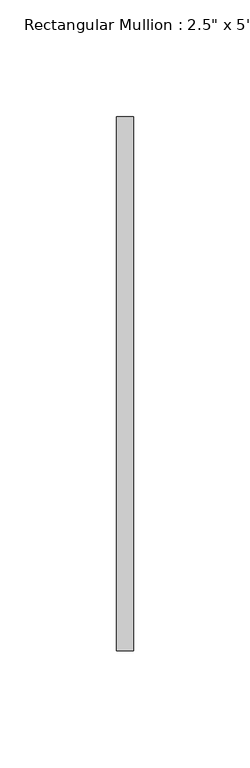
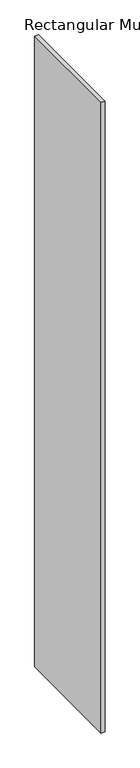
"""IFC4 building model written with IfcOpenShell, lengths in millimetres: member geometry."""

from ifc_helpers import new_model, si_unit, frame, origin, place, context, project, spatial, polyline, outline, extrude, source, transform, mapped, element, save


def member_9e0b9b87(model_context):
    return source(origin(), model_context, "Body", "SweptSolid", [
        extrude(outline(polyline([(0.0, 114.3), (0.0, -114.3), (-7.239, -114.3), (-7.239, 114.3), (0.0, 114.3)])), frame((0.0, 0.0, -1322.6415), z_axis=(0.0, 0.0, 1.0), x_axis=(1.0, 0.0, 0.0)), (0.0, 0.0, 1.0), 1322.6415),
    ])


if __name__ == "__main__":
    model = new_model("IFC4")
    model_context = context("Model", 3, world=origin())
    ifc_project = project(units=[si_unit("LENGTHUNIT", "METRE", prefix="MILLI")], contexts=[model_context])
    site = spatial("IfcSite", under=ifc_project)
    building = spatial("IfcBuilding", under=site)
    placement = place(None, origin())
    member_shape = member_9e0b9b87(model_context)
    element("IfcMember", 1, ObjectType="Rectangular Mullion : 2.5\" x 5\" rectangular", at=placement, inside=building, context=model_context, shape_type="MappedRepresentation", body=[
        mapped(member_shape, transform((0.0, 0.0, 0.0), x_axis=(1.0, 0.0, 0.0), y_axis=(0.0, 1.0, 0.0), z_axis=(0.0, 0.0, 1.0))),
    ])
    save(model, "model.ifc")

# Revit data of these elements
# Type "Rectangular Mullion : 2.5\" x 5\" rectangular"
#   built-in parameter 1007304 = 0.75 (stored number, unit not read)
#   built-in parameter 1007301 = 0.011875 (stored number, unit not read)
#   built-in parameter 1007300 = 0.011875 (stored number, unit not read)
# Element 1 (IfcMember, "Rectangular Mullion : 2.5\" x 5\" rectangular")
#   Materials on its faces: "WINDOW GLASS MATERIAL"
# Materials
#   "WINDOW GLASS MATERIAL": class "Generic", colour RGB 120 120 120, transparency 0, Cost = 0
